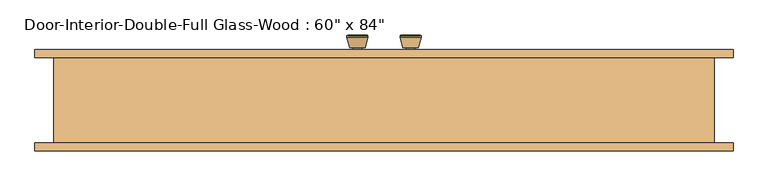
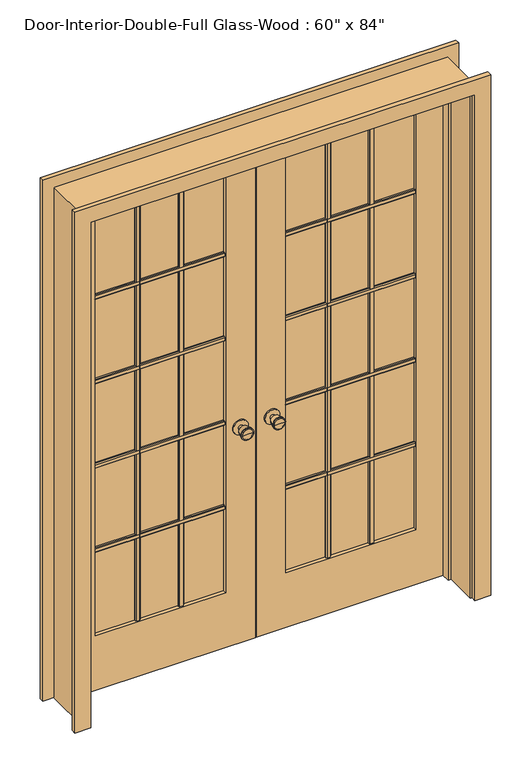
"""IFC4 building model written with IfcOpenShell, lengths in millimetres: door geometry."""

from ifc_helpers import new_model, si_unit, point, frame, frame_2d, origin, place, context, project, spatial, polyline, circle_curve, trimmed, segment, composite_curve, outline, extrude, faceted_brep, source, transform, mapped, element, save
from ifc_brep_helpers import plane_surface, cylinder_surface, revolved_surface, advanced_brep


def door_15ec6cad(model_context):
    return source(origin(), model_context, "Body", "SolidModel", [
        advanced_brep(
        [(-63.5, 104.425, 914.4), (-73.5, 104.425, 914.4), (-53.5, 104.425, 914.4), (-83.9758676, 153.425, 914.4), (-63.5, 153.425, 914.4), (-43.0241324, 153.425, 914.4), (-88.5, 151.5971319, 914.4), (-38.5, 151.5971319, 914.4), (-88.5, 148.1334537, 914.4), (-38.5, 148.1334537, 914.4), (-82.136236, 123.425, 914.4), (-44.863764, 123.425, 914.4), (-73.5, 123.425, 914.4), (-53.5, 123.425, 914.4)],
        [
            (0, 1),
            (1, 2, circle_curve(frame((-63.5, 104.425, 914.4), z_axis=(0.0, -1.0, 0.0), x_axis=(1.0, 0.0, 0.0)), 10.0)),
            (2, 0),
            (2, 1, circle_curve(frame((-63.5, 104.425, 914.4), z_axis=(0.0, -1.0, 0.0), x_axis=(1.0, 0.0, 0.0)), 10.0)),
            (3, 4),
            (4, 5),
            (5, 3, circle_curve(frame((-63.5, 153.425, 914.4), z_axis=(0.0, 1.0, 0.0), x_axis=(1.0, 0.0, 0.0)), 20.4758676)),
            (3, 5, circle_curve(frame((-63.5, 153.425, 914.4), z_axis=(0.0, 1.0, 0.0), x_axis=(1.0, 0.0, 0.0)), 20.4758676)),
            (6, 3),
            (5, 7),
            (7, 6, circle_curve(frame((-63.5, 151.5971319, 914.4), z_axis=(0.0, 1.0, 0.0), x_axis=(1.0, 0.0, 0.0)), 25.0)),
            (6, 7, circle_curve(frame((-63.5, 151.5971319, 914.4), z_axis=(0.0, 1.0, 0.0), x_axis=(1.0, 0.0, 0.0)), 25.0)),
            (8, 6),
            (7, 9),
            (9, 8, circle_curve(frame((-63.5, 148.1334537, 914.4), z_axis=(0.0, 1.0, 0.0), x_axis=(1.0, 0.0, 0.0)), 25.0)),
            (8, 9, circle_curve(frame((-63.5, 148.1334537, 914.4), z_axis=(0.0, 1.0, 0.0), x_axis=(1.0, 0.0, 0.0)), 25.0)),
            (10, 8),
            (9, 11),
            (11, 10, circle_curve(frame((-63.5, 123.425, 914.4), z_axis=(0.0, 1.0, 0.0), x_axis=(1.0, 0.0, 0.0)), 18.636236)),
            (10, 11, circle_curve(frame((-63.5, 123.425, 914.4), z_axis=(0.0, 1.0, 0.0), x_axis=(1.0, 0.0, 0.0)), 18.636236)),
            (12, 10),
            (11, 13),
            (13, 12, circle_curve(frame((-63.5, 123.425, 914.4), z_axis=(0.0, 1.0, 0.0), x_axis=(1.0, 0.0, 0.0)), 10.0)),
            (12, 13, circle_curve(frame((-63.5, 123.425, 914.4), z_axis=(0.0, 1.0, 0.0), x_axis=(1.0, 0.0, 0.0)), 10.0)),
            (1, 12),
            (13, 2),
        ],
        [
            plane_surface(frame((-63.5, 104.425, 914.4), z_axis=(0.0, -1.0, 0.0), x_axis=(1.0, 0.0, 0.0))),
            plane_surface(frame((-63.5, 153.425, 914.4), z_axis=(0.0, 1.0, 0.0), x_axis=(1.0, 0.0, 0.0))),
            revolved_surface(polyline([(-43.0241324, 153.425, 914.4), (-38.5, 151.5971319, 914.4)]), (-63.5, 104.425, 914.4), (0.0, -1.0, 0.0)),
            cylinder_surface(frame((-63.5, 104.425, 914.4), z_axis=(0.0, -1.0, 0.0), x_axis=(1.0, 0.0, 0.0)), 25.0),
            revolved_surface(polyline([(-38.5, 148.1334537, 914.4), (-44.863764, 123.425, 914.4)]), (-63.5, 104.425, 914.4), (0.0, -1.0, 0.0)),
            plane_surface(frame((-63.5, 123.425, 914.4), z_axis=(0.0, -1.0, 0.0), x_axis=(1.0, 0.0, 0.0))),
            cylinder_surface(frame((-63.5, 104.425, 914.4), z_axis=(0.0, -1.0, 0.0), x_axis=(1.0, 0.0, 0.0)), 10.0),
        ],
        [
            (0, [[1, 2, 3]]),
            (0, [[-3, 4, -1]]),
            (1, [[5, 6, 7]]),
            (1, [[-6, -5, 8]]),
            (2, [[9, -7, 10, 11]]),
            (2, [[-10, -8, -9, 12]]),
            (3, [[13, -11, 14, 15]]),
            (3, [[-14, -12, -13, 16]]),
            (4, [[17, -15, 18, 19]]),
            (4, [[-18, -16, -17, 20]]),
            (5, [[21, -19, 22, 23]]),
            (5, [[-22, -20, -21, 24]]),
            (6, [[25, -23, 26, -2]]),
            (6, [[-26, -24, -25, -4]]),
        ],
    ),
        extrude(outline(composite_curve([segment(trimmed(circle_curve(frame_2d((914.4, -63.5)), 30.0), [point((914.4, -33.5))], [point((914.4, -93.5))], False, "CARTESIAN"), True, "CONTINUOUS"), segment(trimmed(circle_curve(frame_2d((914.4, -63.5)), 30.0), [point((914.4, -93.5))], [point((914.4, -33.5))], False, "CARTESIAN"), True, "CONTINUOUS")], self_intersect=False)), frame((0.0, 98.425, 0.0), z_axis=(0.0, 1.0, 0.0), x_axis=(0.0, 0.0, 1.0)), (0.0, 0.0, 1.0), 6.0),
        advanced_brep(
        [(-63.5, 57.5, 914.4), (-53.5, 57.5, 914.4), (-73.5, 57.5, 914.4), (-83.9758676, 8.5, 914.4), (-43.0241324, 8.5, 914.4), (-63.5, 8.5, 914.4), (-88.5, 10.3278681, 914.4), (-38.5, 10.3278681, 914.4), (-88.5, 13.7915463, 914.4), (-38.5, 13.7915463, 914.4), (-82.136236, 38.5, 914.4), (-44.863764, 38.5, 914.4), (-73.5, 38.5, 914.4), (-53.5, 38.5, 914.4)],
        [
            (0, 1),
            (1, 2, circle_curve(frame((-63.5, 57.5, 914.4), z_axis=(0.0, 1.0, 0.0), x_axis=(1.0, 0.0, 0.0)), 10.0)),
            (2, 0),
            (2, 1, circle_curve(frame((-63.5, 57.5, 914.4), z_axis=(0.0, 1.0, 0.0), x_axis=(1.0, 0.0, 0.0)), 10.0)),
            (3, 4, circle_curve(frame((-63.5, 8.5, 914.4), z_axis=(0.0, -1.0, 0.0), x_axis=(1.0, 0.0, 0.0)), 20.4758676)),
            (4, 5),
            (5, 3),
            (4, 3, circle_curve(frame((-63.5, 8.5, 914.4), z_axis=(0.0, -1.0, 0.0), x_axis=(1.0, 0.0, 0.0)), 20.4758676)),
            (6, 7, circle_curve(frame((-63.5, 10.3278681, 914.4), z_axis=(0.0, -1.0, 0.0), x_axis=(1.0, 0.0, 0.0)), 25.0)),
            (7, 4),
            (3, 6),
            (7, 6, circle_curve(frame((-63.5, 10.3278681, 914.4), z_axis=(0.0, -1.0, 0.0), x_axis=(1.0, 0.0, 0.0)), 25.0)),
            (8, 9, circle_curve(frame((-63.5, 13.7915463, 914.4), z_axis=(0.0, -1.0, 0.0), x_axis=(1.0, 0.0, 0.0)), 25.0)),
            (9, 7),
            (6, 8),
            (9, 8, circle_curve(frame((-63.5, 13.7915463, 914.4), z_axis=(0.0, -1.0, 0.0), x_axis=(1.0, 0.0, 0.0)), 25.0)),
            (10, 11, circle_curve(frame((-63.5, 38.5, 914.4), z_axis=(0.0, -1.0, 0.0), x_axis=(1.0, 0.0, 0.0)), 18.636236)),
            (11, 9),
            (8, 10),
            (11, 10, circle_curve(frame((-63.5, 38.5, 914.4), z_axis=(0.0, -1.0, 0.0), x_axis=(1.0, 0.0, 0.0)), 18.636236)),
            (12, 13, circle_curve(frame((-63.5, 38.5, 914.4), z_axis=(0.0, -1.0, 0.0), x_axis=(1.0, 0.0, 0.0)), 10.0)),
            (13, 11),
            (10, 12),
            (13, 12, circle_curve(frame((-63.5, 38.5, 914.4), z_axis=(0.0, -1.0, 0.0), x_axis=(1.0, 0.0, 0.0)), 10.0)),
            (1, 13),
            (12, 2),
        ],
        [
            plane_surface(frame((-63.5, 57.5, 914.4), z_axis=(0.0, 1.0, 0.0), x_axis=(1.0, 0.0, 0.0))),
            plane_surface(frame((-63.5, 8.5, 914.4), z_axis=(0.0, -1.0, 0.0), x_axis=(1.0, 0.0, 0.0))),
            revolved_surface(polyline([(-43.0241324, 8.5, 914.4), (-38.5, 10.3278681, 914.4)]), (-63.5, 57.5, 914.4), (0.0, 1.0, 0.0)),
            cylinder_surface(frame((-63.5, 57.5, 914.4), z_axis=(0.0, 1.0, 0.0), x_axis=(1.0, 0.0, 0.0)), 25.0),
            revolved_surface(polyline([(-38.5, 13.7915463, 914.4), (-44.863764, 38.5, 914.4)]), (-63.5, 57.5, 914.4), (0.0, 1.0, 0.0)),
            plane_surface(frame((-63.5, 38.5, 914.4), z_axis=(0.0, 1.0, 0.0), x_axis=(1.0, 0.0, 0.0))),
            cylinder_surface(frame((-63.5, 57.5, 914.4), z_axis=(0.0, 1.0, 0.0), x_axis=(1.0, 0.0, 0.0)), 10.0),
        ],
        [
            (0, [[1, 2, 3]]),
            (0, [[-3, 4, -1]]),
            (1, [[5, 6, 7]]),
            (1, [[8, -7, -6]]),
            (2, [[9, 10, -5, 11]]),
            (2, [[12, -11, -8, -10]]),
            (3, [[13, 14, -9, 15]]),
            (3, [[16, -15, -12, -14]]),
            (4, [[17, 18, -13, 19]]),
            (4, [[20, -19, -16, -18]]),
            (5, [[21, 22, -17, 23]]),
            (5, [[24, -23, -20, -22]]),
            (6, [[-2, 25, -21, 26]]),
            (6, [[-4, -26, -24, -25]]),
        ],
    ),
        extrude(outline(composite_curve([segment(trimmed(circle_curve(frame_2d((914.4, -63.5)), 30.0), [point((914.4, -33.5))], [point((914.4, -93.5))], False, "CARTESIAN"), True, "CONTINUOUS"), segment(trimmed(circle_curve(frame_2d((914.4, -63.5)), 30.0), [point((914.4, -93.5))], [point((914.4, -33.5))], False, "CARTESIAN"), True, "CONTINUOUS")], self_intersect=False)), frame((0.0, 57.5, 0.0), z_axis=(0.0, 1.0, 0.0), x_axis=(0.0, 0.0, 1.0)), (0.0, 0.0, 1.0), 6.0),
        extrude(outline(polyline([(77.47, 1667.51), (77.47, 1648.46), (71.12, 1648.46), (67.945, 1651.635), (67.945, 1664.335), (71.12, 1667.51), (77.47, 1667.51)])), frame((120.65, 0.0, 0.0), z_axis=(1.0, 0.0, 0.0), x_axis=(0.0, 1.0, 0.0)), (0.0, 0.0, 1.0), 520.7),
        extrude(outline(polyline([(77.47, 1310.9575), (77.47, 1291.9075), (71.12, 1291.9075), (67.945, 1295.0825), (67.945, 1307.7825), (71.12, 1310.9575), (77.47, 1310.9575)])), frame((120.65, 0.0, 0.0), z_axis=(1.0, 0.0, 0.0), x_axis=(0.0, 1.0, 0.0)), (0.0, 0.0, 1.0), 520.7),
        extrude(outline(polyline([(77.47, 954.405), (77.47, 935.355), (71.12, 935.355), (67.945, 938.53), (67.945, 951.23), (71.12, 954.405), (77.47, 954.405)])), frame((120.65, 0.0, 0.0), z_axis=(1.0, 0.0, 0.0), x_axis=(0.0, 1.0, 0.0)), (0.0, 0.0, 1.0), 520.7),
        extrude(outline(polyline([(77.47, 597.8525), (77.47, 578.8025), (71.12, 578.8025), (67.945, 581.9775), (67.945, 594.6775), (71.12, 597.8525), (77.47, 597.8525)])), frame((120.65, 0.0, 0.0), z_axis=(1.0, 0.0, 0.0), x_axis=(0.0, 1.0, 0.0)), (0.0, 0.0, 1.0), 520.7),
        extrude(outline(polyline([(458.2583333, 77.47), (477.3083333, 77.47), (477.3083333, 71.12), (474.1333333, 67.945), (461.4333333, 67.945), (458.2583333, 71.12), (458.2583333, 77.47)])), frame((0.0, 0.0, 231.775), z_axis=(0.0, 0.0, 1.0), x_axis=(1.0, 0.0, 0.0)), (0.0, 0.0, 1.0), 1782.7625),
        extrude(outline(polyline([(284.6916667, 77.47), (303.7416667, 77.47), (303.7416667, 71.12), (300.5666667, 67.945), (287.8666667, 67.945), (284.6916667, 71.12), (284.6916667, 77.47)])), frame((0.0, 0.0, 231.775), z_axis=(0.0, 0.0, 1.0), x_axis=(1.0, 0.0, 0.0)), (0.0, 0.0, 1.0), 1782.7625),
        extrude(outline(polyline([(84.455, 1667.51), (90.805, 1667.51), (93.98, 1664.335), (93.98, 1651.635), (90.805, 1648.46), (84.455, 1648.46), (84.455, 1667.51)])), frame((-641.35, 0.0, 0.0), z_axis=(1.0, 0.0, 0.0), x_axis=(0.0, 1.0, 0.0)), (0.0, 0.0, 1.0), 520.7),
        extrude(outline(polyline([(84.455, 1310.9575), (90.805, 1310.9575), (93.98, 1307.7825), (93.98, 1295.0825), (90.805, 1291.9075), (84.455, 1291.9075), (84.455, 1310.9575)])), frame((-641.35, 0.0, 0.0), z_axis=(1.0, 0.0, 0.0), x_axis=(0.0, 1.0, 0.0)), (0.0, 0.0, 1.0), 520.7),
        extrude(outline(polyline([(84.455, 954.405), (90.805, 954.405), (93.98, 951.23), (93.98, 938.53), (90.805, 935.355), (84.455, 935.355), (84.455, 954.405)])), frame((-641.35, 0.0, 0.0), z_axis=(1.0, 0.0, 0.0), x_axis=(0.0, 1.0, 0.0)), (0.0, 0.0, 1.0), 520.7),
        extrude(outline(polyline([(84.455, 597.8525), (90.805, 597.8525), (93.98, 594.6775), (93.98, 581.9775), (90.805, 578.8025), (84.455, 578.8025), (84.455, 597.8525)])), frame((-641.35, 0.0, 0.0), z_axis=(1.0, 0.0, 0.0), x_axis=(0.0, 1.0, 0.0)), (0.0, 0.0, 1.0), 520.7),
        extrude(outline(polyline([(-303.7416667, 84.455), (-303.7416667, 90.805), (-300.5666667, 93.98), (-287.8666667, 93.98), (-284.6916667, 90.805), (-284.6916667, 84.455), (-303.7416667, 84.455)])), frame((0.0, 0.0, 231.775), z_axis=(0.0, 0.0, 1.0), x_axis=(1.0, 0.0, 0.0)), (0.0, 0.0, 1.0), 1782.7625),
        extrude(outline(polyline([(-477.3083333, 84.455), (-477.3083333, 90.805), (-474.1333333, 93.98), (-461.4333333, 93.98), (-458.2583333, 90.805), (-458.2583333, 84.455), (-477.3083333, 84.455)])), frame((0.0, 0.0, 231.775), z_axis=(0.0, 0.0, 1.0), x_axis=(1.0, 0.0, 0.0)), (0.0, 0.0, 1.0), 1782.7625),
        extrude(outline(polyline([(84.455, 1667.51), (90.805, 1667.51), (93.98, 1664.335), (93.98, 1651.635), (90.805, 1648.46), (84.455, 1648.46), (84.455, 1667.51)])), frame((120.65, 0.0, 0.0), z_axis=(1.0, 0.0, 0.0), x_axis=(0.0, 1.0, 0.0)), (0.0, 0.0, 1.0), 520.7),
        extrude(outline(polyline([(84.455, 1310.9575), (90.805, 1310.9575), (93.98, 1307.7825), (93.98, 1295.0825), (90.805, 1291.9075), (84.455, 1291.9075), (84.455, 1310.9575)])), frame((120.65, 0.0, 0.0), z_axis=(1.0, 0.0, 0.0), x_axis=(0.0, 1.0, 0.0)), (0.0, 0.0, 1.0), 520.7),
        extrude(outline(polyline([(84.455, 954.405), (90.805, 954.405), (93.98, 951.23), (93.98, 938.53), (90.805, 935.355), (84.455, 935.355), (84.455, 954.405)])), frame((120.65, 0.0, 0.0), z_axis=(1.0, 0.0, 0.0), x_axis=(0.0, 1.0, 0.0)), (0.0, 0.0, 1.0), 520.7),
        extrude(outline(polyline([(84.455, 597.8525), (90.805, 597.8525), (93.98, 594.6775), (93.98, 581.9775), (90.805, 578.8025), (84.455, 578.8025), (84.455, 597.8525)])), frame((120.65, 0.0, 0.0), z_axis=(1.0, 0.0, 0.0), x_axis=(0.0, 1.0, 0.0)), (0.0, 0.0, 1.0), 520.7),
        extrude(outline(polyline([(458.2583333, 84.455), (458.2583333, 90.805), (461.4333333, 93.98), (474.1333333, 93.98), (477.3083333, 90.805), (477.3083333, 84.455), (458.2583333, 84.455)])), frame((0.0, 0.0, 231.775), z_axis=(0.0, 0.0, 1.0), x_axis=(1.0, 0.0, 0.0)), (0.0, 0.0, 1.0), 1782.7625),
        extrude(outline(polyline([(284.6916667, 84.455), (284.6916667, 90.805), (287.8666667, 93.98), (300.5666667, 93.98), (303.7416667, 90.805), (303.7416667, 84.455), (284.6916667, 84.455)])), frame((0.0, 0.0, 231.775), z_axis=(0.0, 0.0, 1.0), x_axis=(1.0, 0.0, 0.0)), (0.0, 0.0, 1.0), 1782.7625),
        extrude(outline(polyline([(77.47, 1667.51), (77.47, 1648.46), (71.12, 1648.46), (67.945, 1651.635), (67.945, 1664.335), (71.12, 1667.51), (77.47, 1667.51)])), frame((-641.35, 0.0, 0.0), z_axis=(1.0, 0.0, 0.0), x_axis=(0.0, 1.0, 0.0)), (0.0, 0.0, 1.0), 520.7),
        extrude(outline(polyline([(77.47, 1310.9575), (77.47, 1291.9075), (71.12, 1291.9075), (67.945, 1295.0825), (67.945, 1307.7825), (71.12, 1310.9575), (77.47, 1310.9575)])), frame((-641.35, 0.0, 0.0), z_axis=(1.0, 0.0, 0.0), x_axis=(0.0, 1.0, 0.0)), (0.0, 0.0, 1.0), 520.7),
        extrude(outline(polyline([(77.47, 954.405), (77.47, 935.355), (71.12, 935.355), (67.945, 938.53), (67.945, 951.23), (71.12, 954.405), (77.47, 954.405)])), frame((-641.35, 0.0, 0.0), z_axis=(1.0, 0.0, 0.0), x_axis=(0.0, 1.0, 0.0)), (0.0, 0.0, 1.0), 520.7),
        extrude(outline(polyline([(77.47, 597.8525), (77.47, 578.8025), (71.12, 578.8025), (67.945, 581.9775), (67.945, 594.6775), (71.12, 597.8525), (77.47, 597.8525)])), frame((-641.35, 0.0, 0.0), z_axis=(1.0, 0.0, 0.0), x_axis=(0.0, 1.0, 0.0)), (0.0, 0.0, 1.0), 520.7),
        extrude(outline(polyline([(-303.7416667, 77.47), (-284.6916667, 77.47), (-284.6916667, 71.12), (-287.8666667, 67.945), (-300.5666667, 67.945), (-303.7416667, 71.12), (-303.7416667, 77.47)])), frame((0.0, 0.0, 231.775), z_axis=(0.0, 0.0, 1.0), x_axis=(1.0, 0.0, 0.0)), (0.0, 0.0, 1.0), 1782.7625),
        extrude(outline(polyline([(-477.3083333, 77.47), (-458.2583333, 77.47), (-458.2583333, 71.12), (-461.4333333, 67.945), (-474.1333333, 67.945), (-477.3083333, 71.12), (-477.3083333, 77.47)])), frame((0.0, 0.0, 231.775), z_axis=(0.0, 0.0, 1.0), x_axis=(1.0, 0.0, 0.0)), (0.0, 0.0, 1.0), 1782.7625),
        advanced_brep(
        [(63.5, 57.5, 914.4), (73.5, 57.5, 914.4), (53.5, 57.5, 914.4), (83.9758676, 8.5, 914.4), (63.5, 8.5, 914.4), (43.0241324, 8.5, 914.4), (88.5, 10.3278681, 914.4), (38.5, 10.3278681, 914.4), (88.5, 13.7915463, 914.4), (38.5, 13.7915463, 914.4), (82.136236, 38.5, 914.4), (44.863764, 38.5, 914.4), (73.5, 38.5, 914.4), (53.5, 38.5, 914.4)],
        [
            (0, 1),
            (1, 2, circle_curve(frame((63.5, 57.5, 914.4), z_axis=(0.0, 1.0, 0.0), x_axis=(-1.0, 0.0, 0.0)), 10.0)),
            (2, 0),
            (2, 1, circle_curve(frame((63.5, 57.5, 914.4), z_axis=(0.0, 1.0, 0.0), x_axis=(-1.0, 0.0, 0.0)), 10.0)),
            (3, 4),
            (4, 5),
            (5, 3, circle_curve(frame((63.5, 8.5, 914.4), z_axis=(0.0, -1.0, 0.0), x_axis=(-1.0, 0.0, 0.0)), 20.4758676)),
            (3, 5, circle_curve(frame((63.5, 8.5, 914.4), z_axis=(0.0, -1.0, 0.0), x_axis=(-1.0, 0.0, 0.0)), 20.4758676)),
            (6, 3),
            (5, 7),
            (7, 6, circle_curve(frame((63.5, 10.3278681, 914.4), z_axis=(0.0, -1.0, 0.0), x_axis=(-1.0, 0.0, 0.0)), 25.0)),
            (6, 7, circle_curve(frame((63.5, 10.3278681, 914.4), z_axis=(0.0, -1.0, 0.0), x_axis=(-1.0, 0.0, 0.0)), 25.0)),
            (8, 6),
            (7, 9),
            (9, 8, circle_curve(frame((63.5, 13.7915463, 914.4), z_axis=(0.0, -1.0, 0.0), x_axis=(-1.0, 0.0, 0.0)), 25.0)),
            (8, 9, circle_curve(frame((63.5, 13.7915463, 914.4), z_axis=(0.0, -1.0, 0.0), x_axis=(-1.0, 0.0, 0.0)), 25.0)),
            (10, 8),
            (9, 11),
            (11, 10, circle_curve(frame((63.5, 38.5, 914.4), z_axis=(0.0, -1.0, 0.0), x_axis=(-1.0, 0.0, 0.0)), 18.636236)),
            (10, 11, circle_curve(frame((63.5, 38.5, 914.4), z_axis=(0.0, -1.0, 0.0), x_axis=(-1.0, 0.0, 0.0)), 18.636236)),
            (12, 10),
            (11, 13),
            (13, 12, circle_curve(frame((63.5, 38.5, 914.4), z_axis=(0.0, -1.0, 0.0), x_axis=(-1.0, 0.0, 0.0)), 10.0)),
            (12, 13, circle_curve(frame((63.5, 38.5, 914.4), z_axis=(0.0, -1.0, 0.0), x_axis=(-1.0, 0.0, 0.0)), 10.0)),
            (1, 12),
            (13, 2),
        ],
        [
            plane_surface(frame((63.5, 57.5, 914.4), z_axis=(0.0, 1.0, 0.0), x_axis=(-1.0, 0.0, 0.0))),
            plane_surface(frame((63.5, 8.5, 914.4), z_axis=(0.0, -1.0, 0.0), x_axis=(-1.0, 0.0, 0.0))),
            revolved_surface(polyline([(43.0241324, 8.5, 914.4), (38.5, 10.3278681, 914.4)]), (63.5, 57.5, 914.4), (0.0, 1.0, 0.0)),
            cylinder_surface(frame((63.5, 57.5, 914.4), z_axis=(0.0, 1.0, 0.0), x_axis=(-1.0, 0.0, 0.0)), 25.0),
            revolved_surface(polyline([(38.5, 13.7915463, 914.4), (44.863764, 38.5, 914.4)]), (63.5, 57.5, 914.4), (0.0, 1.0, 0.0)),
            plane_surface(frame((63.5, 38.5, 914.4), z_axis=(0.0, 1.0, 0.0), x_axis=(-1.0, 0.0, 0.0))),
            cylinder_surface(frame((63.5, 57.5, 914.4), z_axis=(0.0, 1.0, 0.0), x_axis=(-1.0, 0.0, 0.0)), 10.0),
        ],
        [
            (0, [[1, 2, 3]]),
            (0, [[-3, 4, -1]]),
            (1, [[5, 6, 7]]),
            (1, [[-6, -5, 8]]),
            (2, [[9, -7, 10, 11]]),
            (2, [[-10, -8, -9, 12]]),
            (3, [[13, -11, 14, 15]]),
            (3, [[-14, -12, -13, 16]]),
            (4, [[17, -15, 18, 19]]),
            (4, [[-18, -16, -17, 20]]),
            (5, [[21, -19, 22, 23]]),
            (5, [[-22, -20, -21, 24]]),
            (6, [[25, -23, 26, -2]]),
            (6, [[-26, -24, -25, -4]]),
        ],
    ),
        extrude(outline(composite_curve([segment(trimmed(circle_curve(frame_2d((914.4, 63.5)), 30.0), [point((914.4, 33.5))], [point((914.4, 93.5))], False, "CARTESIAN"), True, "CONTINUOUS"), segment(trimmed(circle_curve(frame_2d((914.4, 63.5)), 30.0), [point((914.4, 93.5))], [point((914.4, 33.5))], False, "CARTESIAN"), True, "CONTINUOUS")], self_intersect=False)), frame((0.0, 57.5, 0.0), z_axis=(0.0, 1.0, 0.0), x_axis=(0.0, 0.0, 1.0)), (0.0, 0.0, 1.0), 6.0),
        advanced_brep(
        [(63.5, 104.425, 914.4), (53.5, 104.425, 914.4), (73.5, 104.425, 914.4), (83.9758676, 153.425, 914.4), (43.0241324, 153.425, 914.4), (63.5, 153.425, 914.4), (88.5, 151.5971319, 914.4), (38.5, 151.5971319, 914.4), (88.5, 148.1334537, 914.4), (38.5, 148.1334537, 914.4), (82.136236, 123.425, 914.4), (44.863764, 123.425, 914.4), (73.5, 123.425, 914.4), (53.5, 123.425, 914.4)],
        [
            (0, 1),
            (1, 2, circle_curve(frame((63.5, 104.425, 914.4), z_axis=(0.0, -1.0, 0.0), x_axis=(-1.0, 0.0, 0.0)), 10.0)),
            (2, 0),
            (2, 1, circle_curve(frame((63.5, 104.425, 914.4), z_axis=(0.0, -1.0, 0.0), x_axis=(-1.0, 0.0, 0.0)), 10.0)),
            (3, 4, circle_curve(frame((63.5, 153.425, 914.4), z_axis=(0.0, 1.0, 0.0), x_axis=(-1.0, 0.0, 0.0)), 20.4758676)),
            (4, 5),
            (5, 3),
            (4, 3, circle_curve(frame((63.5, 153.425, 914.4), z_axis=(0.0, 1.0, 0.0), x_axis=(-1.0, 0.0, 0.0)), 20.4758676)),
            (6, 7, circle_curve(frame((63.5, 151.5971319, 914.4), z_axis=(0.0, 1.0, 0.0), x_axis=(-1.0, 0.0, 0.0)), 25.0)),
            (7, 4),
            (3, 6),
            (7, 6, circle_curve(frame((63.5, 151.5971319, 914.4), z_axis=(0.0, 1.0, 0.0), x_axis=(-1.0, 0.0, 0.0)), 25.0)),
            (8, 9, circle_curve(frame((63.5, 148.1334537, 914.4), z_axis=(0.0, 1.0, 0.0), x_axis=(-1.0, 0.0, 0.0)), 25.0)),
            (9, 7),
            (6, 8),
            (9, 8, circle_curve(frame((63.5, 148.1334537, 914.4), z_axis=(0.0, 1.0, 0.0), x_axis=(-1.0, 0.0, 0.0)), 25.0)),
            (10, 11, circle_curve(frame((63.5, 123.425, 914.4), z_axis=(0.0, 1.0, 0.0), x_axis=(-1.0, 0.0, 0.0)), 18.636236)),
            (11, 9),
            (8, 10),
            (11, 10, circle_curve(frame((63.5, 123.425, 914.4), z_axis=(0.0, 1.0, 0.0), x_axis=(-1.0, 0.0, 0.0)), 18.636236)),
            (12, 13, circle_curve(frame((63.5, 123.425, 914.4), z_axis=(0.0, 1.0, 0.0), x_axis=(-1.0, 0.0, 0.0)), 10.0)),
            (13, 11),
            (10, 12),
            (13, 12, circle_curve(frame((63.5, 123.425, 914.4), z_axis=(0.0, 1.0, 0.0), x_axis=(-1.0, 0.0, 0.0)), 10.0)),
            (1, 13),
            (12, 2),
        ],
        [
            plane_surface(frame((63.5, 104.425, 914.4), z_axis=(0.0, -1.0, 0.0), x_axis=(-1.0, 0.0, 0.0))),
            plane_surface(frame((63.5, 153.425, 914.4), z_axis=(0.0, 1.0, 0.0), x_axis=(-1.0, 0.0, 0.0))),
            revolved_surface(polyline([(43.0241324, 153.425, 914.4), (38.5, 151.5971319, 914.4)]), (63.5, 104.425, 914.4), (0.0, -1.0, 0.0)),
            cylinder_surface(frame((63.5, 104.425, 914.4), z_axis=(0.0, -1.0, 0.0), x_axis=(-1.0, 0.0, 0.0)), 25.0),
            revolved_surface(polyline([(38.5, 148.1334537, 914.4), (44.863764, 123.425, 914.4)]), (63.5, 104.425, 914.4), (0.0, -1.0, 0.0)),
            plane_surface(frame((63.5, 123.425, 914.4), z_axis=(0.0, -1.0, 0.0), x_axis=(-1.0, 0.0, 0.0))),
            cylinder_surface(frame((63.5, 104.425, 914.4), z_axis=(0.0, -1.0, 0.0), x_axis=(-1.0, 0.0, 0.0)), 10.0),
        ],
        [
            (0, [[1, 2, 3]]),
            (0, [[-3, 4, -1]]),
            (1, [[5, 6, 7]]),
            (1, [[8, -7, -6]]),
            (2, [[9, 10, -5, 11]]),
            (2, [[12, -11, -8, -10]]),
            (3, [[13, 14, -9, 15]]),
            (3, [[16, -15, -12, -14]]),
            (4, [[17, 18, -13, 19]]),
            (4, [[20, -19, -16, -18]]),
            (5, [[21, 22, -17, 23]]),
            (5, [[24, -23, -20, -22]]),
            (6, [[-2, 25, -21, 26]]),
            (6, [[-4, -26, -24, -25]]),
        ],
    ),
        extrude(outline(composite_curve([segment(trimmed(circle_curve(frame_2d((914.4, 63.5)), 30.0), [point((914.4, 33.5))], [point((914.4, 93.5))], False, "CARTESIAN"), True, "CONTINUOUS"), segment(trimmed(circle_curve(frame_2d((914.4, 63.5)), 30.0), [point((914.4, 93.5))], [point((914.4, 33.5))], False, "CARTESIAN"), True, "CONTINUOUS")], self_intersect=False)), frame((0.0, 98.425, 0.0), z_axis=(0.0, 1.0, 0.0), x_axis=(0.0, 0.0, 1.0)), (0.0, 0.0, 1.0), 6.0),
        extrude(outline(polyline([(0.0, 768.35), (0.0, 831.85), (2203.45, 831.85), (2203.45, -831.85), (0.0, -831.85), (0.0, -768.35), (2139.95, -768.35), (2139.95, 768.35), (0.0, 768.35)])), frame((0.0, 98.425, 0.0), z_axis=(0.0, 1.0, 0.0), x_axis=(0.0, 0.0, 1.0)), (0.0, 0.0, 1.0), 19.05),
        extrude(outline(polyline([(0.0, 768.35), (0.0, 831.85), (2203.45, 831.85), (2203.45, -831.85), (0.0, -831.85), (0.0, -768.35), (2139.95, -768.35), (2139.95, 768.35), (0.0, 768.35)])), frame((0.0, -123.825, 0.0), z_axis=(0.0, 1.0, 0.0), x_axis=(0.0, 0.0, 1.0)), (0.0, 0.0, 1.0), 19.05),
        extrude(outline(polyline([(2133.6, -762.0), (0.0, -762.0), (0.0, -1.6019111), (2133.6, -1.6019111), (2133.6, -762.0)]), holes=[polyline([(231.775, -641.35), (2014.5375, -641.35), (2014.5375, -120.65), (231.775, -120.65), (231.775, -641.35)])]), frame((0.0, 63.5, 0.0), z_axis=(0.0, 1.0, 0.0), x_axis=(0.0, 0.0, 1.0)), (0.0, 0.0, 1.0), 34.925),
        extrude(outline(polyline([(0.0, 762.0), (2133.6, 762.0), (2133.6, 1.5875), (0.0, 1.5875), (0.0, 762.0)]), holes=[polyline([(2014.5375, 120.65), (2014.5375, 641.35), (231.775, 641.35), (231.775, 120.65), (2014.5375, 120.65)])]), frame((0.0, 63.5, 0.0), z_axis=(0.0, 1.0, 0.0), x_axis=(0.0, 0.0, 1.0)), (0.0, 0.0, 1.0), 34.925),
        faceted_brep([(787.4, 98.425, 0.0), (787.4, -104.775, 0.0), (762.0, -104.775, 0.0), (762.0, 28.575, 0.0), (749.3, 28.575, 0.0), (749.3, 63.5, 0.0), (762.0, 63.5, 0.0), (762.0, 98.425, 0.0), (787.4, 98.425, 2159.0), (787.4, -104.775, 2159.0), (-787.4, -104.775, 2159.0), (-787.4, -104.775, 0.0), (-762.0, -104.775, 0.0), (-762.0, -104.775, 2133.6), (762.0, -104.775, 2133.6), (762.0, 28.575, 2133.6), (-762.0, 28.575, 2133.6), (-762.0, 28.575, 0.0), (-749.3, 28.575, 0.0), (-749.3, 28.575, 2120.9), (749.3, 28.575, 2120.9), (749.3, 63.5, 2120.9), (1.5875, 63.5, 2120.9), (-1.6019111, 63.5, 2120.9), (-749.3, 63.5, 2120.9), (-749.3, 63.5, 0.0), (-762.0, 63.5, 0.0), (-762.0, 63.5, 2133.6), (-1.6019111, 63.5, 2133.6), (1.5875, 63.5, 2133.6), (762.0, 63.5, 2133.6), (762.0, 98.425, 2133.6), (1.5875, 98.425, 2133.6), (-1.6019111, 98.425, 2133.6), (-762.0, 98.425, 2133.6), (-762.0, 98.425, 0.0), (-787.4, 98.425, 0.0), (-787.4, 98.425, 2159.0)], [[[0, 1, 2, 3, 4, 5, 6, 7]], [[1, 0, 8, 9]], [[2, 1, 9, 10, 11, 12, 13, 14]], [[3, 2, 14, 15]], [[4, 3, 15, 16, 17, 18, 19, 20]], [[5, 4, 20, 21]], [[6, 5, 21, 22, 23, 24, 25, 26, 27, 28, 29, 30]], [[7, 6, 30, 31]], [[0, 7, 31, 32, 33, 34, 35, 36, 37, 8]], [[9, 8, 37, 10]], [[14, 13, 16, 15]], [[20, 19, 24, 23, 22, 21]], [[31, 30, 29, 28, 27, 34, 33, 32]], [[12, 11, 36, 35, 26, 25, 18, 17]], [[11, 10, 37, 36]], [[13, 12, 17, 16]], [[19, 18, 25, 24]], [[27, 26, 35, 34]]]),
        extrude(outline(polyline([(641.35, 77.47), (120.65, 77.47), (120.65, 84.455), (641.35, 84.455), (641.35, 77.47)])), frame((0.0, 0.0, 231.775), z_axis=(0.0, 0.0, 1.0), x_axis=(1.0, 0.0, 0.0)), (0.0, 0.0, 1.0), 1782.7625),
        extrude(outline(polyline([(-120.65, 77.47), (-641.35, 77.47), (-641.35, 84.455), (-120.65, 84.455), (-120.65, 77.47)])), frame((0.0, 0.0, 231.775), z_axis=(0.0, 0.0, 1.0), x_axis=(1.0, 0.0, 0.0)), (0.0, 0.0, 1.0), 1782.7625),
    ])


if __name__ == "__main__":
    model = new_model("IFC4")
    model_context = context("Model", 3, world=origin())
    ifc_project = project(units=[si_unit("LENGTHUNIT", "METRE", prefix="MILLI")], contexts=[model_context])
    site = spatial("IfcSite", under=ifc_project)
    building = spatial("IfcBuilding", under=site)
    placement = place(None, origin())
    door_shape = door_15ec6cad(model_context)
    element("IfcDoor", 1, ObjectType="Door-Interior-Double-Full Glass-Wood : 60\" x 84\"", at=placement, inside=building, context=model_context, shape_type="MappedRepresentation", body=[
        mapped(door_shape, transform((0.0, 0.0, 0.0), x_axis=(1.0, 0.0, 0.0), y_axis=(0.0, 1.0, 0.0), z_axis=(0.0, 0.0, 1.0))),
    ])
    save(model, "model.ifc")

# Revit data of these elements
# Type "Door-Interior-Double-Full Glass-Wood : 60\" x 84\""
#   Type Mark = "9"
#   Assembly Code = "C1020300"
#   Analytic Construction = "French door, wood frame with single glass"
#   Top Rail = 0' - 4 11/16"
#   Thickness = 0' - 1 3/8"
#   Thermal Resistance (R) = 1.0696 (h·ft²·°F)/BTU
#   Swing Angle [instance default] = 90.00°
#   Stiles = 0' - 4 3/4"
#   Rough Width = 5' - 2"
#   Rough Height = 7' - 1"
#   Panel Width = 2' - 6"
#   Height = 7' - 0"
#   Width = 5' - 0"
#   Heat Transfer Coefficient (U) = 0.9350 BTU/(h·ft²·°F)
#   Bottom Rail = 0' - 9 1/8"
#   Show Grill [instance default] = yes
#   Trim Material = Cherry
#   Panel Material = Cherry
#   Frame Material = Cherry
#   Door Handle Material = Aluminum
#   Visual Light Transmittance = 0
#   Solar Heat Gain Coefficient = 0
#   Wall Closure = (empty or 0)
#   Function = (empty or 0)
# Element 1 (IfcDoor, "Door-Interior-Double-Full Glass-Wood : 60\" x 84\"")
#   Materials on its faces: "Cherry", "Aluminum", "Glass"
# Materials
#   "Cherry": class "Wood", colour RGB 226 177 128, transparency 0, Description = "Prunus Serotina", Cost = 0
#   "Aluminum": class "Metal", colour RGB 247 247 247, transparency 0, Description = "Aluminum 6061", Cost = 0
#   "Glass": class "Glass", colour RGB 0 128 192, transparency 0.75, Description = "Soda Lime Glass", Cost = 0
